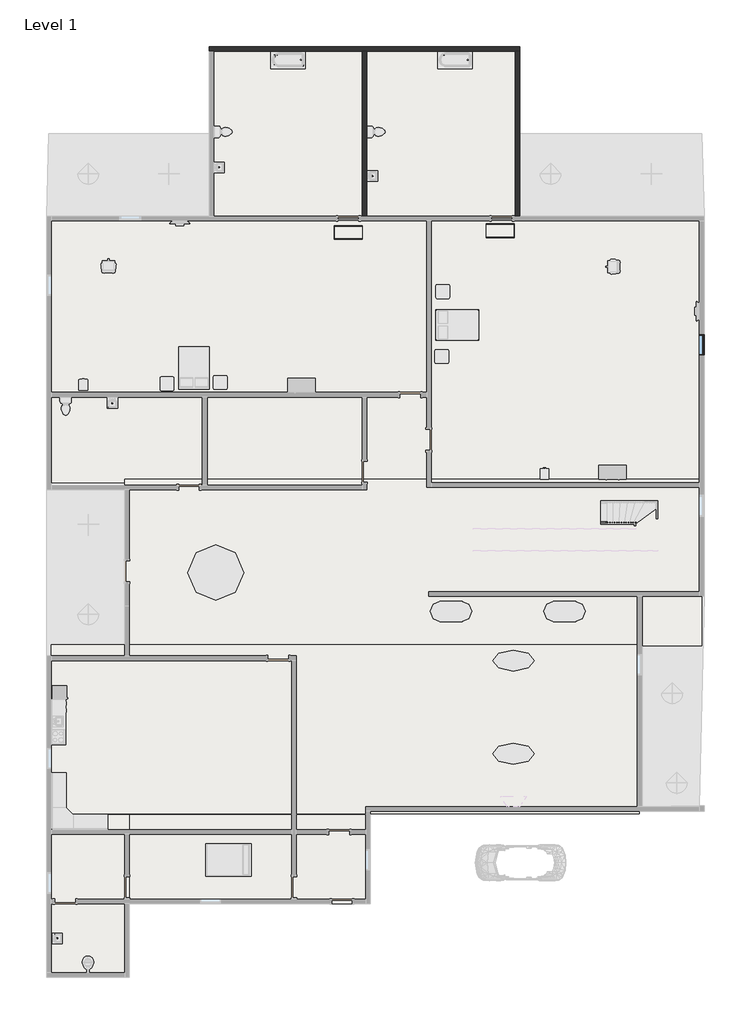
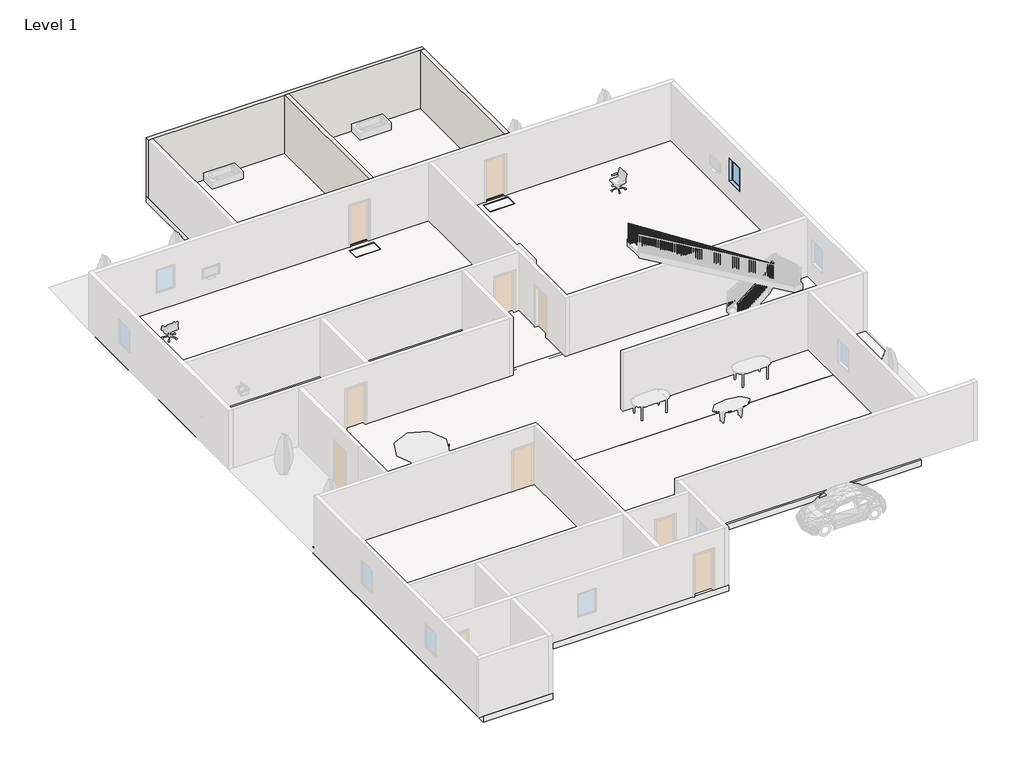
# One storey, part 2 of 4: 7 slabs, 3 walls, 1 railing, 1 window.
"""IFC4 building model written with IfcOpenShell, lengths in millimetres."""

from ifc_helpers import new_model, si_unit, frame, origin, origin_with_axes, place, context, project, spatial, polyline, outline, extrude, faceted_brep, transform, mapped, element, save
from components import window_e2841890

model = new_model("IFC4")

# Units and contexts
model_context = context("Model", 3, world=origin())
ifc_project = project(units=[si_unit("LENGTHUNIT", "METRE", prefix="MILLI")], contexts=[model_context])

# Site, building, storey
site = spatial("IfcSite", under=ifc_project)
building = spatial("IfcBuilding", under=site)
storey = spatial("IfcBuildingStorey", under=building, Name="Level 1", Elevation=0.0)

# Railing
placement = place(None, origin())
element("IfcRailing", 1, ObjectType="Handrail - Rectangular", at=placement, inside=storey, context=model_context, shape_type="SolidModel", body=[
    faceted_brep([(11576.2992414, 107.8275916, 1025.2529681), (11576.2992414, 107.8275916, 959.7067088), (11576.2992414, 57.0275916, 959.7067088), (11576.2992414, 57.0275916, 1025.2529681), (13027.8309332, 107.8275916, 2208.7848338), (13078.6309332, 107.8275916, 2184.659247), (13078.6309332, 57.0275916, 2184.659247), (13027.8309332, 57.0275916, 2208.7848338), (13027.8309332, 107.8275916, 2414.6281882), (13078.6309332, 107.8275916, 2363.8281882), (13078.6309332, 57.0275916, 2363.8281882), (13027.8309332, 57.0275916, 2414.6281882), (13154.8309332, 107.8275916, 2414.6281882), (13154.8309332, 107.8275916, 2363.8281882), (13104.0309332, 57.0275916, 2363.8281882), (13104.0309332, 57.0275916, 2414.6281882), (13154.8309332, -19.1724084, 2414.6281882), (13154.8309332, -48.2937422, 2363.8281882), (13104.0309332, -48.2937422, 2363.8281882), (13104.0309332, -19.1724084, 2414.6281882), (13154.8309332, -146.1724084, 2631.5051451), (13154.8309332, -196.9724084, 2617.7256424), (13104.0309332, -196.9724084, 2617.7256424), (13104.0309332, -146.1724084, 2631.5051451), (13154.8309332, -146.1724084, 2824.6954835), (13154.8309332, -196.9724084, 2773.8954835), (13104.0309332, -196.9724084, 2773.8954835), (13104.0309332, -146.1724084, 2824.6954835), (13154.8309332, -273.1724084, 2824.6954835), (13154.8309332, -273.1724084, 2773.8954835), (13104.0309332, -222.3724084, 2773.8954835), (13104.0309332, -222.3724084, 2824.6954835), (13027.8309332, -273.1724084, 2824.6954835), (13012.8842088, -273.1724084, 2773.8954835), (13012.8842088, -222.3724084, 2773.8954835), (13027.8309332, -222.3724084, 2824.6954835), (5988.2992414, -273.1724084, 7359.7294681), (5988.2992414, -222.3724084, 7359.7294681), (5988.2992414, -222.3724084, 7299.3004322), (5988.2992414, -273.1724084, 7299.3004322)], [[[0, 1, 2, 3]], [[1, 0, 4, 5]], [[2, 1, 5, 6]], [[3, 2, 6, 7]], [[0, 3, 7, 4]], [[5, 4, 8, 9]], [[6, 5, 9, 10]], [[7, 6, 10, 11]], [[4, 7, 11, 8]], [[9, 8, 12, 13]], [[10, 9, 13, 14]], [[11, 10, 14, 15]], [[8, 11, 15, 12]], [[13, 12, 16, 17]], [[14, 13, 17, 18]], [[15, 14, 18, 19]], [[12, 15, 19, 16]], [[17, 16, 20, 21]], [[18, 17, 21, 22]], [[19, 18, 22, 23]], [[16, 19, 23, 20]], [[21, 20, 24, 25]], [[22, 21, 25, 26]], [[23, 22, 26, 27]], [[20, 23, 27, 24]], [[25, 24, 28, 29]], [[26, 25, 29, 30]], [[27, 26, 30, 31]], [[24, 27, 31, 28]], [[29, 28, 32, 33]], [[30, 29, 33, 34]], [[31, 30, 34, 35]], [[28, 31, 35, 32]], [[36, 37, 38, 39]], [[33, 32, 36, 39]], [[34, 33, 39, 38]], [[35, 34, 38, 37]], [[32, 35, 37, 36]]]),
    extrude(outline(polyline([(7231.8259142, 6093.0369367), (7244.098378, 6073.9869367), (6265.3333333, 6073.9869367), (6265.3333333, 6093.0369367), (7231.8259142, 6093.0369367)])), frame((0.0, -257.2974084, 0.0), z_axis=(0.0, 1.0, 0.0), x_axis=(0.0, 0.0, 1.0)), (0.0, 0.0, 1.0), 19.05),
    extrude(outline(polyline([(7166.3727743, 6194.6369367), (7178.645238, 6175.5869367), (6265.3333333, 6175.5869367), (6265.3333333, 6194.6369367), (7166.3727743, 6194.6369367)])), frame((0.0, -257.2974084, 0.0), z_axis=(0.0, 1.0, 0.0), x_axis=(0.0, 0.0, 1.0)), (0.0, 0.0, 1.0), 19.05),
    extrude(outline(polyline([(7100.9196344, 6296.2369367), (7113.1920981, 6277.1869367), (6096.0, 6277.1869367), (6096.0, 6296.2369367), (7100.9196344, 6296.2369367)])), frame((0.0, -257.2974084, 0.0), z_axis=(0.0, 1.0, 0.0), x_axis=(0.0, 0.0, 1.0)), (0.0, 0.0, 1.0), 19.05),
    extrude(outline(polyline([(7035.4664945, 6397.8369367), (7047.7389582, 6378.7869367), (6096.0, 6378.7869367), (6096.0, 6397.8369367), (7035.4664945, 6397.8369367)])), frame((0.0, -257.2974084, 0.0), z_axis=(0.0, 1.0, 0.0), x_axis=(0.0, 0.0, 1.0)), (0.0, 0.0, 1.0), 19.05),
    extrude(outline(polyline([(6970.0133545, 6499.4369367), (6982.2858183, 6480.3869367), (6096.0, 6480.3869367), (6096.0, 6499.4369367), (6970.0133545, 6499.4369367)])), frame((0.0, -257.2974084, 0.0), z_axis=(0.0, 1.0, 0.0), x_axis=(0.0, 0.0, 1.0)), (0.0, 0.0, 1.0), 19.05),
    extrude(outline(polyline([(6904.5602146, 6601.0369367), (6916.8326783, 6581.9869367), (5926.6666667, 6581.9869367), (5926.6666667, 6601.0369367), (6904.5602146, 6601.0369367)])), frame((0.0, -257.2974084, 0.0), z_axis=(0.0, 1.0, 0.0), x_axis=(0.0, 0.0, 1.0)), (0.0, 0.0, 1.0), 19.05),
    extrude(outline(polyline([(6839.1070747, 6702.6369367), (6851.3795384, 6683.5869367), (5926.6666667, 6683.5869367), (5926.6666667, 6702.6369367), (6839.1070747, 6702.6369367)])), frame((0.0, -257.2974084, 0.0), z_axis=(0.0, 1.0, 0.0), x_axis=(0.0, 0.0, 1.0)), (0.0, 0.0, 1.0), 19.05),
    extrude(outline(polyline([(6773.6539348, 6804.2369367), (6785.9263985, 6785.1869367), (5926.6666667, 6785.1869367), (5926.6666667, 6804.2369367), (6773.6539348, 6804.2369367)])), frame((0.0, -257.2974084, 0.0), z_axis=(0.0, 1.0, 0.0), x_axis=(0.0, 0.0, 1.0)), (0.0, 0.0, 1.0), 19.05),
    extrude(outline(polyline([(6708.2007948, 6905.8369367), (6720.4732586, 6886.7869367), (5757.3333333, 6886.7869367), (5757.3333333, 6905.8369367), (6708.2007948, 6905.8369367)])), frame((0.0, -257.2974084, 0.0), z_axis=(0.0, 1.0, 0.0), x_axis=(0.0, 0.0, 1.0)), (0.0, 0.0, 1.0), 19.05),
    extrude(outline(polyline([(6642.7476549, 7007.4369367), (6655.0201186, 6988.3869367), (5757.3333333, 6988.3869367), (5757.3333333, 7007.4369367), (6642.7476549, 7007.4369367)])), frame((0.0, -257.2974084, 0.0), z_axis=(0.0, 1.0, 0.0), x_axis=(0.0, 0.0, 1.0)), (0.0, 0.0, 1.0), 19.05),
    extrude(outline(polyline([(6577.294515, 7109.0369367), (6589.5669787, 7089.9869367), (5757.3333333, 7089.9869367), (5757.3333333, 7109.0369367), (6577.294515, 7109.0369367)])), frame((0.0, -257.2974084, 0.0), z_axis=(0.0, 1.0, 0.0), x_axis=(0.0, 0.0, 1.0)), (0.0, 0.0, 1.0), 19.05),
    extrude(outline(polyline([(6511.8413751, 7210.6369367), (6524.1138388, 7191.5869367), (5588.0, 7191.5869367), (5588.0, 7210.6369367), (6511.8413751, 7210.6369367)])), frame((0.0, -257.2974084, 0.0), z_axis=(0.0, 1.0, 0.0), x_axis=(0.0, 0.0, 1.0)), (0.0, 0.0, 1.0), 19.05),
    extrude(outline(polyline([(6446.3882351, 7312.2369367), (6458.6606989, 7293.1869367), (5588.0, 7293.1869367), (5588.0, 7312.2369367), (6446.3882351, 7312.2369367)])), frame((0.0, -257.2974084, 0.0), z_axis=(0.0, 1.0, 0.0), x_axis=(0.0, 0.0, 1.0)), (0.0, 0.0, 1.0), 19.05),
    extrude(outline(polyline([(6380.9350952, 7413.8369367), (6393.2075589, 7394.7869367), (5418.6666667, 7394.7869367), (5418.6666667, 7413.8369367), (6380.9350952, 7413.8369367)])), frame((0.0, -257.2974084, 0.0), z_axis=(0.0, 1.0, 0.0), x_axis=(0.0, 0.0, 1.0)), (0.0, 0.0, 1.0), 19.05),
    extrude(outline(polyline([(6315.4819553, 7515.4369367), (6327.754419, 7496.3869367), (5418.6666667, 7496.3869367), (5418.6666667, 7515.4369367), (6315.4819553, 7515.4369367)])), frame((0.0, -257.2974084, 0.0), z_axis=(0.0, 1.0, 0.0), x_axis=(0.0, 0.0, 1.0)), (0.0, 0.0, 1.0), 19.05),
    extrude(outline(polyline([(6250.0288153, 7617.0369367), (6262.3012791, 7597.9869367), (5418.6666667, 7597.9869367), (5418.6666667, 7617.0369367), (6250.0288153, 7617.0369367)])), frame((0.0, -257.2974084, 0.0), z_axis=(0.0, 1.0, 0.0), x_axis=(0.0, 0.0, 1.0)), (0.0, 0.0, 1.0), 19.05),
    extrude(outline(polyline([(6184.5756754, 7718.6369367), (6196.8481392, 7699.5869367), (5249.3333333, 7699.5869367), (5249.3333333, 7718.6369367), (6184.5756754, 7718.6369367)])), frame((0.0, -257.2974084, 0.0), z_axis=(0.0, 1.0, 0.0), x_axis=(0.0, 0.0, 1.0)), (0.0, 0.0, 1.0), 19.05),
    extrude(outline(polyline([(6119.1225355, 7820.2369367), (6131.3949992, 7801.1869367), (5249.3333333, 7801.1869367), (5249.3333333, 7820.2369367), (6119.1225355, 7820.2369367)])), frame((0.0, -257.2974084, 0.0), z_axis=(0.0, 1.0, 0.0), x_axis=(0.0, 0.0, 1.0)), (0.0, 0.0, 1.0), 19.05),
    extrude(outline(polyline([(6053.6693956, 7921.8369367), (6065.9418593, 7902.7869367), (5249.3333333, 7902.7869367), (5249.3333333, 7921.8369367), (6053.6693956, 7921.8369367)])), frame((0.0, -257.2974084, 0.0), z_axis=(0.0, 1.0, 0.0), x_axis=(0.0, 0.0, 1.0)), (0.0, 0.0, 1.0), 19.05),
    extrude(outline(polyline([(5988.2162556, 8023.4369367), (6000.4887194, 8004.3869367), (5080.0, 8004.3869367), (5080.0, 8023.4369367), (5988.2162556, 8023.4369367)])), frame((0.0, -257.2974084, 0.0), z_axis=(0.0, 1.0, 0.0), x_axis=(0.0, 0.0, 1.0)), (0.0, 0.0, 1.0), 19.05),
    extrude(outline(polyline([(5922.7631157, 8125.0369367), (5935.0355795, 8105.9869367), (5080.0, 8105.9869367), (5080.0, 8125.0369367), (5922.7631157, 8125.0369367)])), frame((0.0, -257.2974084, 0.0), z_axis=(0.0, 1.0, 0.0), x_axis=(0.0, 0.0, 1.0)), (0.0, 0.0, 1.0), 19.05),
    extrude(outline(polyline([(5857.3099758, 8226.6369367), (5869.5824395, 8207.5869367), (5080.0, 8207.5869367), (5080.0, 8226.6369367), (5857.3099758, 8226.6369367)])), frame((0.0, -257.2974084, 0.0), z_axis=(0.0, 1.0, 0.0), x_axis=(0.0, 0.0, 1.0)), (0.0, 0.0, 1.0), 19.05),
    extrude(outline(polyline([(5791.8568359, 8328.2369367), (5804.1292996, 8309.1869367), (4910.6666667, 8309.1869367), (4910.6666667, 8328.2369367), (5791.8568359, 8328.2369367)])), frame((0.0, -257.2974084, 0.0), z_axis=(0.0, 1.0, 0.0), x_axis=(0.0, 0.0, 1.0)), (0.0, 0.0, 1.0), 19.05),
    extrude(outline(polyline([(5726.4036959, 8429.8369367), (5738.6761597, 8410.7869367), (4910.6666667, 8410.7869367), (4910.6666667, 8429.8369367), (5726.4036959, 8429.8369367)])), frame((0.0, -257.2974084, 0.0), z_axis=(0.0, 1.0, 0.0), x_axis=(0.0, 0.0, 1.0)), (0.0, 0.0, 1.0), 19.05),
    extrude(outline(polyline([(5660.950556, 8531.4369367), (5673.2230198, 8512.3869367), (4741.3333333, 8512.3869367), (4741.3333333, 8531.4369367), (5660.950556, 8531.4369367)])), frame((0.0, -257.2974084, 0.0), z_axis=(0.0, 1.0, 0.0), x_axis=(0.0, 0.0, 1.0)), (0.0, 0.0, 1.0), 19.05),
    extrude(outline(polyline([(5595.4974161, 8633.0369367), (5607.7698798, 8613.9869367), (4741.3333333, 8613.9869367), (4741.3333333, 8633.0369367), (5595.4974161, 8633.0369367)])), frame((0.0, -257.2974084, 0.0), z_axis=(0.0, 1.0, 0.0), x_axis=(0.0, 0.0, 1.0)), (0.0, 0.0, 1.0), 19.05),
    extrude(outline(polyline([(5530.0442762, 8734.6369367), (5542.3167399, 8715.5869367), (4741.3333333, 8715.5869367), (4741.3333333, 8734.6369367), (5530.0442762, 8734.6369367)])), frame((0.0, -257.2974084, 0.0), z_axis=(0.0, 1.0, 0.0), x_axis=(0.0, 0.0, 1.0)), (0.0, 0.0, 1.0), 19.05),
    extrude(outline(polyline([(5464.5911362, 8836.2369367), (5476.8636, 8817.1869367), (4572.0, 8817.1869367), (4572.0, 8836.2369367), (5464.5911362, 8836.2369367)])), frame((0.0, -257.2974084, 0.0), z_axis=(0.0, 1.0, 0.0), x_axis=(0.0, 0.0, 1.0)), (0.0, 0.0, 1.0), 19.05),
    extrude(outline(polyline([(5399.1379963, 8937.8369367), (5411.41046, 8918.7869367), (4572.0, 8918.7869367), (4572.0, 8937.8369367), (5399.1379963, 8937.8369367)])), frame((0.0, -257.2974084, 0.0), z_axis=(0.0, 1.0, 0.0), x_axis=(0.0, 0.0, 1.0)), (0.0, 0.0, 1.0), 19.05),
    extrude(outline(polyline([(5333.6848564, 9039.4369367), (5345.9573201, 9020.3869367), (4572.0, 9020.3869367), (4572.0, 9039.4369367), (5333.6848564, 9039.4369367)])), frame((0.0, -257.2974084, 0.0), z_axis=(0.0, 1.0, 0.0), x_axis=(0.0, 0.0, 1.0)), (0.0, 0.0, 1.0), 19.05),
    extrude(outline(polyline([(5268.2317165, 9141.0369367), (5280.5041802, 9121.9869367), (4402.6666667, 9121.9869367), (4402.6666667, 9141.0369367), (5268.2317165, 9141.0369367)])), frame((0.0, -257.2974084, 0.0), z_axis=(0.0, 1.0, 0.0), x_axis=(0.0, 0.0, 1.0)), (0.0, 0.0, 1.0), 19.05),
    extrude(outline(polyline([(5202.7785765, 9242.6369367), (5215.0510403, 9223.5869367), (4402.6666667, 9223.5869367), (4402.6666667, 9242.6369367), (5202.7785765, 9242.6369367)])), frame((0.0, -257.2974084, 0.0), z_axis=(0.0, 1.0, 0.0), x_axis=(0.0, 0.0, 1.0)), (0.0, 0.0, 1.0), 19.05),
    extrude(outline(polyline([(5137.3254366, 9344.2369367), (5149.5979003, 9325.1869367), (4233.3333333, 9325.1869367), (4233.3333333, 9344.2369367), (5137.3254366, 9344.2369367)])), frame((0.0, -257.2974084, 0.0), z_axis=(0.0, 1.0, 0.0), x_axis=(0.0, 0.0, 1.0)), (0.0, 0.0, 1.0), 19.05),
    extrude(outline(polyline([(5071.8722967, 9445.8369367), (5084.1447604, 9426.7869367), (4233.3333333, 9426.7869367), (4233.3333333, 9445.8369367), (5071.8722967, 9445.8369367)])), frame((0.0, -257.2974084, 0.0), z_axis=(0.0, 1.0, 0.0), x_axis=(0.0, 0.0, 1.0)), (0.0, 0.0, 1.0), 19.05),
    extrude(outline(polyline([(5006.4191568, 9547.4369367), (5018.6916205, 9528.3869367), (4233.3333333, 9528.3869367), (4233.3333333, 9547.4369367), (5006.4191568, 9547.4369367)])), frame((0.0, -257.2974084, 0.0), z_axis=(0.0, 1.0, 0.0), x_axis=(0.0, 0.0, 1.0)), (0.0, 0.0, 1.0), 19.05),
    extrude(outline(polyline([(4940.9660168, 9649.0369367), (4953.2384806, 9629.9869367), (4064.0, 9629.9869367), (4064.0, 9649.0369367), (4940.9660168, 9649.0369367)])), frame((0.0, -257.2974084, 0.0), z_axis=(0.0, 1.0, 0.0), x_axis=(0.0, 0.0, 1.0)), (0.0, 0.0, 1.0), 19.05),
    extrude(outline(polyline([(4875.5128769, 9750.6369367), (4887.7853406, 9731.5869367), (4064.0, 9731.5869367), (4064.0, 9750.6369367), (4875.5128769, 9750.6369367)])), frame((0.0, -257.2974084, 0.0), z_axis=(0.0, 1.0, 0.0), x_axis=(0.0, 0.0, 1.0)), (0.0, 0.0, 1.0), 19.05),
    extrude(outline(polyline([(4810.059737, 9852.2369367), (4822.3322007, 9833.1869367), (4064.0, 9833.1869367), (4064.0, 9852.2369367), (4810.059737, 9852.2369367)])), frame((0.0, -257.2974084, 0.0), z_axis=(0.0, 1.0, 0.0), x_axis=(0.0, 0.0, 1.0)), (0.0, 0.0, 1.0), 19.05),
    extrude(outline(polyline([(4744.6065971, 9953.8369367), (4756.8790608, 9934.7869367), (3894.6666667, 9934.7869367), (3894.6666667, 9953.8369367), (4744.6065971, 9953.8369367)])), frame((0.0, -257.2974084, 0.0), z_axis=(0.0, 1.0, 0.0), x_axis=(0.0, 0.0, 1.0)), (0.0, 0.0, 1.0), 19.05),
    extrude(outline(polyline([(4679.1534571, 10055.4369367), (4691.4259209, 10036.3869367), (3894.6666667, 10036.3869367), (3894.6666667, 10055.4369367), (4679.1534571, 10055.4369367)])), frame((0.0, -257.2974084, 0.0), z_axis=(0.0, 1.0, 0.0), x_axis=(0.0, 0.0, 1.0)), (0.0, 0.0, 1.0), 19.05),
    extrude(outline(polyline([(4613.7003172, 10157.0369367), (4625.9727809, 10137.9869367), (3894.6666667, 10137.9869367), (3894.6666667, 10157.0369367), (4613.7003172, 10157.0369367)])), frame((0.0, -257.2974084, 0.0), z_axis=(0.0, 1.0, 0.0), x_axis=(0.0, 0.0, 1.0)), (0.0, 0.0, 1.0), 19.05),
    extrude(outline(polyline([(4548.2471773, 10258.6369367), (4560.519641, 10239.5869367), (3725.3333333, 10239.5869367), (3725.3333333, 10258.6369367), (4548.2471773, 10258.6369367)])), frame((0.0, -257.2974084, 0.0), z_axis=(0.0, 1.0, 0.0), x_axis=(0.0, 0.0, 1.0)), (0.0, 0.0, 1.0), 19.05),
    extrude(outline(polyline([(4482.7940373, 10360.2369367), (4495.0665011, 10341.1869367), (3725.3333333, 10341.1869367), (3725.3333333, 10360.2369367), (4482.7940373, 10360.2369367)])), frame((0.0, -257.2974084, 0.0), z_axis=(0.0, 1.0, 0.0), x_axis=(0.0, 0.0, 1.0)), (0.0, 0.0, 1.0), 19.05),
    extrude(outline(polyline([(4417.3408974, 10461.8369367), (4429.6133612, 10442.7869367), (3556.0, 10442.7869367), (3556.0, 10461.8369367), (4417.3408974, 10461.8369367)])), frame((0.0, -257.2974084, 0.0), z_axis=(0.0, 1.0, 0.0), x_axis=(0.0, 0.0, 1.0)), (0.0, 0.0, 1.0), 19.05),
    extrude(outline(polyline([(4351.8877575, 10563.4369367), (4364.1602212, 10544.3869367), (3556.0, 10544.3869367), (3556.0, 10563.4369367), (4351.8877575, 10563.4369367)])), frame((0.0, -257.2974084, 0.0), z_axis=(0.0, 1.0, 0.0), x_axis=(0.0, 0.0, 1.0)), (0.0, 0.0, 1.0), 19.05),
    extrude(outline(polyline([(4286.4346176, 10665.0369367), (4298.7070813, 10645.9869367), (3556.0, 10645.9869367), (3556.0, 10665.0369367), (4286.4346176, 10665.0369367)])), frame((0.0, -257.2974084, 0.0), z_axis=(0.0, 1.0, 0.0), x_axis=(0.0, 0.0, 1.0)), (0.0, 0.0, 1.0), 19.05),
    extrude(outline(polyline([(4220.9814776, 10766.6369367), (4233.2539414, 10747.5869367), (3386.6666667, 10747.5869367), (3386.6666667, 10766.6369367), (4220.9814776, 10766.6369367)])), frame((0.0, -257.2974084, 0.0), z_axis=(0.0, 1.0, 0.0), x_axis=(0.0, 0.0, 1.0)), (0.0, 0.0, 1.0), 19.05),
    extrude(outline(polyline([(4155.5283377, 10868.2369367), (4167.8008015, 10849.1869367), (3386.6666667, 10849.1869367), (3386.6666667, 10868.2369367), (4155.5283377, 10868.2369367)])), frame((0.0, -257.2974084, 0.0), z_axis=(0.0, 1.0, 0.0), x_axis=(0.0, 0.0, 1.0)), (0.0, 0.0, 1.0), 19.05),
    extrude(outline(polyline([(4090.0751978, 10969.8369367), (4102.3476615, 10950.7869367), (3386.6666667, 10950.7869367), (3386.6666667, 10969.8369367), (4090.0751978, 10969.8369367)])), frame((0.0, -257.2974084, 0.0), z_axis=(0.0, 1.0, 0.0), x_axis=(0.0, 0.0, 1.0)), (0.0, 0.0, 1.0), 19.05),
    extrude(outline(polyline([(4024.6220579, 11071.4369367), (4036.8945216, 11052.3869367), (3217.3333333, 11052.3869367), (3217.3333333, 11071.4369367), (4024.6220579, 11071.4369367)])), frame((0.0, -257.2974084, 0.0), z_axis=(0.0, 1.0, 0.0), x_axis=(0.0, 0.0, 1.0)), (0.0, 0.0, 1.0), 19.05),
    extrude(outline(polyline([(3959.1689179, 11173.0369367), (3971.4413817, 11153.9869367), (3217.3333333, 11153.9869367), (3217.3333333, 11173.0369367), (3959.1689179, 11173.0369367)])), frame((0.0, -257.2974084, 0.0), z_axis=(0.0, 1.0, 0.0), x_axis=(0.0, 0.0, 1.0)), (0.0, 0.0, 1.0), 19.05),
    extrude(outline(polyline([(3893.715778, 11274.6369367), (3905.9882418, 11255.5869367), (3217.3333333, 11255.5869367), (3217.3333333, 11274.6369367), (3893.715778, 11274.6369367)])), frame((0.0, -257.2974084, 0.0), z_axis=(0.0, 1.0, 0.0), x_axis=(0.0, 0.0, 1.0)), (0.0, 0.0, 1.0), 19.05),
    extrude(outline(polyline([(3828.2626381, 11376.2369367), (3840.5351018, 11357.1869367), (3048.0, 11357.1869367), (3048.0, 11376.2369367), (3828.2626381, 11376.2369367)])), frame((0.0, -257.2974084, 0.0), z_axis=(0.0, 1.0, 0.0), x_axis=(0.0, 0.0, 1.0)), (0.0, 0.0, 1.0), 19.05),
    extrude(outline(polyline([(3762.8094982, 11477.8369367), (3775.0819619, 11458.7869367), (3048.0, 11458.7869367), (3048.0, 11477.8369367), (3762.8094982, 11477.8369367)])), frame((0.0, -257.2974084, 0.0), z_axis=(0.0, 1.0, 0.0), x_axis=(0.0, 0.0, 1.0)), (0.0, 0.0, 1.0), 19.05),
    extrude(outline(polyline([(3697.3563582, 11579.4369367), (3709.628822, 11560.3869367), (2878.6666667, 11560.3869367), (2878.6666667, 11579.4369367), (3697.3563582, 11579.4369367)])), frame((0.0, -257.2974084, 0.0), z_axis=(0.0, 1.0, 0.0), x_axis=(0.0, 0.0, 1.0)), (0.0, 0.0, 1.0), 19.05),
    extrude(outline(polyline([(3631.9032183, 11681.0369367), (3644.175682, 11661.9869367), (2878.6666667, 11661.9869367), (2878.6666667, 11681.0369367), (3631.9032183, 11681.0369367)])), frame((0.0, -257.2974084, 0.0), z_axis=(0.0, 1.0, 0.0), x_axis=(0.0, 0.0, 1.0)), (0.0, 0.0, 1.0), 19.05),
    extrude(outline(polyline([(3566.4500784, 11782.6369367), (3578.7225421, 11763.5869367), (2878.6666667, 11763.5869367), (2878.6666667, 11782.6369367), (3566.4500784, 11782.6369367)])), frame((0.0, -257.2974084, 0.0), z_axis=(0.0, 1.0, 0.0), x_axis=(0.0, 0.0, 1.0)), (0.0, 0.0, 1.0), 19.05),
    extrude(outline(polyline([(3500.9969385, 11884.2369367), (3513.2694022, 11865.1869367), (2709.3333333, 11865.1869367), (2709.3333333, 11884.2369367), (3500.9969385, 11884.2369367)])), frame((0.0, -257.2974084, 0.0), z_axis=(0.0, 1.0, 0.0), x_axis=(0.0, 0.0, 1.0)), (0.0, 0.0, 1.0), 19.05),
    extrude(outline(polyline([(3435.5437985, 11985.8369367), (3447.8162623, 11966.7869367), (2709.3333333, 11966.7869367), (2709.3333333, 11985.8369367), (3435.5437985, 11985.8369367)])), frame((0.0, -257.2974084, 0.0), z_axis=(0.0, 1.0, 0.0), x_axis=(0.0, 0.0, 1.0)), (0.0, 0.0, 1.0), 19.05),
    extrude(outline(polyline([(3370.0906586, 12087.4369367), (3382.3631223, 12068.3869367), (2709.3333333, 12068.3869367), (2709.3333333, 12087.4369367), (3370.0906586, 12087.4369367)])), frame((0.0, -257.2974084, 0.0), z_axis=(0.0, 1.0, 0.0), x_axis=(0.0, 0.0, 1.0)), (0.0, 0.0, 1.0), 19.05),
    extrude(outline(polyline([(3304.6375187, 12189.0369367), (3316.9099824, 12169.9869367), (2540.0, 12169.9869367), (2540.0, 12189.0369367), (3304.6375187, 12189.0369367)])), frame((0.0, -257.2974084, 0.0), z_axis=(0.0, 1.0, 0.0), x_axis=(0.0, 0.0, 1.0)), (0.0, 0.0, 1.0), 19.05),
    extrude(outline(polyline([(3239.1843788, 12290.6369367), (3251.4568425, 12271.5869367), (2540.0, 12271.5869367), (2540.0, 12290.6369367), (3239.1843788, 12290.6369367)])), frame((0.0, -257.2974084, 0.0), z_axis=(0.0, 1.0, 0.0), x_axis=(0.0, 0.0, 1.0)), (0.0, 0.0, 1.0), 19.05),
    extrude(outline(polyline([(3173.7312388, 12392.2369367), (3186.0037026, 12373.1869367), (2370.6666667, 12373.1869367), (2370.6666667, 12392.2369367), (3173.7312388, 12392.2369367)])), frame((0.0, -257.2974084, 0.0), z_axis=(0.0, 1.0, 0.0), x_axis=(0.0, 0.0, 1.0)), (0.0, 0.0, 1.0), 19.05),
    extrude(outline(polyline([(3108.2780989, 12493.8369367), (3120.5505626, 12474.7869367), (2370.6666667, 12474.7869367), (2370.6666667, 12493.8369367), (3108.2780989, 12493.8369367)])), frame((0.0, -257.2974084, 0.0), z_axis=(0.0, 1.0, 0.0), x_axis=(0.0, 0.0, 1.0)), (0.0, 0.0, 1.0), 19.05),
    extrude(outline(polyline([(3042.824959, 12595.4369367), (3055.0974227, 12576.3869367), (2370.6666667, 12576.3869367), (2370.6666667, 12595.4369367), (3042.824959, 12595.4369367)])), frame((0.0, -257.2974084, 0.0), z_axis=(0.0, 1.0, 0.0), x_axis=(0.0, 0.0, 1.0)), (0.0, 0.0, 1.0), 19.05),
    extrude(outline(polyline([(2977.3718191, 12697.0369367), (2989.6442828, 12677.9869367), (2201.3333333, 12677.9869367), (2201.3333333, 12697.0369367), (2977.3718191, 12697.0369367)])), frame((0.0, -257.2974084, 0.0), z_axis=(0.0, 1.0, 0.0), x_axis=(0.0, 0.0, 1.0)), (0.0, 0.0, 1.0), 19.05),
    extrude(outline(polyline([(2911.9186791, 12798.6369367), (2924.1911429, 12779.5869367), (2201.3333333, 12779.5869367), (2201.3333333, 12798.6369367), (2911.9186791, 12798.6369367)])), frame((0.0, -257.2974084, 0.0), z_axis=(0.0, 1.0, 0.0), x_axis=(0.0, 0.0, 1.0)), (0.0, 0.0, 1.0), 19.05),
    extrude(outline(polyline([(2846.4655392, 12900.2369367), (2858.7380029, 12881.1869367), (2032.0, 12881.1869367), (2032.0, 12900.2369367), (2846.4655392, 12900.2369367)])), frame((0.0, -257.2974084, 0.0), z_axis=(0.0, 1.0, 0.0), x_axis=(0.0, 0.0, 1.0)), (0.0, 0.0, 1.0), 19.05),
    extrude(outline(polyline([(2781.0123993, 13001.8369367), (2793.284863, 12982.7869367), (2032.0, 12982.7869367), (2032.0, 13001.8369367), (2781.0123993, 13001.8369367)])), frame((0.0, -257.2974084, 0.0), z_axis=(0.0, 1.0, 0.0), x_axis=(0.0, 0.0, 1.0)), (0.0, 0.0, 1.0), 19.05),
    extrude(outline(polyline([(-145.0833121, 2529.115018), (-126.0333121, 2496.5834745), (-126.0333121, 1524.0), (-145.0833121, 1524.0), (-145.0833121, 2529.115018)])), frame((13119.9059332, 0.0, 0.0), z_axis=(1.0, 0.0, 0.0), x_axis=(0.0, 1.0, 0.0)), (0.0, 0.0, 1.0), 19.05),
    extrude(outline(polyline([(-43.4833121, 2355.6134525), (-24.4333121, 2323.0819089), (-24.4333121, 1524.0), (-43.4833121, 1524.0), (-43.4833121, 2355.6134525)])), frame((13119.9059332, 0.0, 0.0), z_axis=(1.0, 0.0, 0.0), x_axis=(0.0, 1.0, 0.0)), (0.0, 0.0, 1.0), 19.05),
    extrude(outline(polyline([(2127.2519138, 13008.2242414), (2111.7191617, 12989.1742414), (1016.0, 12989.1742414), (1016.0, 13008.2242414), (2127.2519138, 13008.2242414)])), frame((0.0, 72.9025916, 0.0), z_axis=(0.0, 1.0, 0.0), x_axis=(0.0, 0.0, 1.0)), (0.0, 0.0, 1.0), 19.05),
    extrude(outline(polyline([(2044.4105689, 12906.6242414), (2028.8778167, 12887.5742414), (1016.0, 12887.5742414), (1016.0, 12906.6242414), (2044.4105689, 12906.6242414)])), frame((0.0, 72.9025916, 0.0), z_axis=(0.0, 1.0, 0.0), x_axis=(0.0, 0.0, 1.0)), (0.0, 0.0, 1.0), 19.05),
    extrude(outline(polyline([(1961.569224, 12805.0242414), (1946.0364718, 12785.9742414), (846.6666667, 12785.9742414), (846.6666667, 12805.0242414), (1961.569224, 12805.0242414)])), frame((0.0, 72.9025916, 0.0), z_axis=(0.0, 1.0, 0.0), x_axis=(0.0, 0.0, 1.0)), (0.0, 0.0, 1.0), 19.05),
    extrude(outline(polyline([(1878.7278791, 12703.4242414), (1863.1951269, 12684.3742414), (846.6666667, 12684.3742414), (846.6666667, 12703.4242414), (1878.7278791, 12703.4242414)])), frame((0.0, 72.9025916, 0.0), z_axis=(0.0, 1.0, 0.0), x_axis=(0.0, 0.0, 1.0)), (0.0, 0.0, 1.0), 19.05),
    extrude(outline(polyline([(1795.8865341, 12601.8242414), (1780.353782, 12582.7742414), (677.3333333, 12582.7742414), (677.3333333, 12601.8242414), (1795.8865341, 12601.8242414)])), frame((0.0, 72.9025916, 0.0), z_axis=(0.0, 1.0, 0.0), x_axis=(0.0, 0.0, 1.0)), (0.0, 0.0, 1.0), 19.05),
    extrude(outline(polyline([(1713.0451892, 12500.2242414), (1697.5124371, 12481.1742414), (677.3333333, 12481.1742414), (677.3333333, 12500.2242414), (1713.0451892, 12500.2242414)])), frame((0.0, 72.9025916, 0.0), z_axis=(0.0, 1.0, 0.0), x_axis=(0.0, 0.0, 1.0)), (0.0, 0.0, 1.0), 19.05),
    extrude(outline(polyline([(1630.2038443, 12398.6242414), (1614.6710921, 12379.5742414), (508.0, 12379.5742414), (508.0, 12398.6242414), (1630.2038443, 12398.6242414)])), frame((0.0, 72.9025916, 0.0), z_axis=(0.0, 1.0, 0.0), x_axis=(0.0, 0.0, 1.0)), (0.0, 0.0, 1.0), 19.05),
    extrude(outline(polyline([(1547.3624994, 12297.0242414), (1531.8297472, 12277.9742414), (508.0, 12277.9742414), (508.0, 12297.0242414), (1547.3624994, 12297.0242414)])), frame((0.0, 72.9025916, 0.0), z_axis=(0.0, 1.0, 0.0), x_axis=(0.0, 0.0, 1.0)), (0.0, 0.0, 1.0), 19.05),
    extrude(outline(polyline([(1464.5211545, 12195.4242414), (1448.9884023, 12176.3742414), (508.0, 12176.3742414), (508.0, 12195.4242414), (1464.5211545, 12195.4242414)])), frame((0.0, 72.9025916, 0.0), z_axis=(0.0, 1.0, 0.0), x_axis=(0.0, 0.0, 1.0)), (0.0, 0.0, 1.0), 19.05),
    extrude(outline(polyline([(1381.6798095, 12093.8242414), (1366.1470574, 12074.7742414), (338.6666667, 12074.7742414), (338.6666667, 12093.8242414), (1381.6798095, 12093.8242414)])), frame((0.0, 72.9025916, 0.0), z_axis=(0.0, 1.0, 0.0), x_axis=(0.0, 0.0, 1.0)), (0.0, 0.0, 1.0), 19.05),
    extrude(outline(polyline([(1298.8384646, 11992.2242414), (1283.3057124, 11973.1742414), (338.6666667, 11973.1742414), (338.6666667, 11992.2242414), (1298.8384646, 11992.2242414)])), frame((0.0, 72.9025916, 0.0), z_axis=(0.0, 1.0, 0.0), x_axis=(0.0, 0.0, 1.0)), (0.0, 0.0, 1.0), 19.05),
    extrude(outline(polyline([(1215.9971197, 11890.6242414), (1200.4643675, 11871.5742414), (338.6666667, 11871.5742414), (338.6666667, 11890.6242414), (1215.9971197, 11890.6242414)])), frame((0.0, 72.9025916, 0.0), z_axis=(0.0, 1.0, 0.0), x_axis=(0.0, 0.0, 1.0)), (0.0, 0.0, 1.0), 19.05),
    extrude(outline(polyline([(1133.1557748, 11789.0242414), (1117.6230226, 11769.9742414), (169.3333333, 11769.9742414), (169.3333333, 11789.0242414), (1133.1557748, 11789.0242414)])), frame((0.0, 72.9025916, 0.0), z_axis=(0.0, 1.0, 0.0), x_axis=(0.0, 0.0, 1.0)), (0.0, 0.0, 1.0), 19.05),
    extrude(outline(polyline([(1050.3144298, 11687.4242414), (1034.7816777, 11668.3742414), (169.3333333, 11668.3742414), (169.3333333, 11687.4242414), (1050.3144298, 11687.4242414)])), frame((0.0, 72.9025916, 0.0), z_axis=(0.0, 1.0, 0.0), x_axis=(0.0, 0.0, 1.0)), (0.0, 0.0, 1.0), 19.05),
    extrude(outline(polyline([(13103.4369367, -238.2474084), (13103.4369367, -257.2974084), (13084.3869367, -257.2974084), (13084.3869367, -238.2474084), (13103.4369367, -238.2474084)])), frame((0.0, 0.0, 1862.6666667), z_axis=(0.0, 0.0, 1.0), x_axis=(1.0, 0.0, 0.0)), (0.0, 0.0, 1.0), 911.2288168),
    extrude(outline(polyline([(13119.9059332, -238.2474084), (13138.9559332, -238.2474084), (13138.9559332, -257.2974084), (13119.9059332, -257.2974084), (13119.9059332, -238.2474084)])), frame((0.0, 0.0, 1862.6666667), z_axis=(0.0, 0.0, 1.0), x_axis=(1.0, 0.0, 0.0)), (0.0, 0.0, 1.0), 911.2288168),
    extrude(outline(polyline([(13119.9059332, -224.8479336), (13138.9559332, -224.8479336), (13138.9559332, -243.8979336), (13119.9059332, -243.8979336), (13119.9059332, -224.8479336)])), frame((0.0, 0.0, 1693.3333333), z_axis=(0.0, 0.0, 1.0), x_axis=(1.0, 0.0, 0.0)), (0.0, 0.0, 1.0), 1080.5621501),
    extrude(outline(polyline([(13119.9059332, 77.1666879), (13138.9559332, 77.1666879), (13138.9559332, 58.1166879), (13119.9059332, 58.1166879), (13119.9059332, 77.1666879)])), frame((0.0, 0.0, 1354.6666667), z_axis=(0.0, 0.0, 1.0), x_axis=(1.0, 0.0, 0.0)), (0.0, 0.0, 1.0), 1009.1615215),
    extrude(outline(polyline([(13119.9059332, 72.9025916), (13119.9059332, 91.9525916), (13138.9559332, 91.9525916), (13138.9559332, 72.9025916), (13119.9059332, 72.9025916)])), frame((0.0, 0.0, 1185.3333333), z_axis=(0.0, 0.0, 1.0), x_axis=(1.0, 0.0, 0.0)), (0.0, 0.0, 1.0), 1178.4948549),
    extrude(outline(polyline([(13088.9385769, 72.9025916), (13088.9385769, 91.9525916), (13107.9885769, 91.9525916), (13107.9885769, 72.9025916), (13088.9385769, 72.9025916)])), frame((0.0, 0.0, 1185.3333333), z_axis=(0.0, 0.0, 1.0), x_axis=(1.0, 0.0, 0.0)), (0.0, 0.0, 1.0), 1178.4948549),
    extrude(outline(polyline([(7287.0279685, 6007.3492414), (7299.3004322, 5988.2992414), (6265.3333333, 5988.2992414), (6265.3333333, 6007.3492414), (7287.0279685, 6007.3492414)])), frame((0.0, -257.2974084, 0.0), z_axis=(0.0, 1.0, 0.0), x_axis=(0.0, 0.0, 1.0)), (0.0, 0.0, 1.0), 19.05),
    extrude(outline(polyline([(975.239461, 11595.3492414), (959.7067088, 11576.2992414), (169.3333333, 11576.2992414), (169.3333333, 11595.3492414), (975.239461, 11595.3492414)])), frame((0.0, 72.9025916, 0.0), z_axis=(0.0, 1.0, 0.0), x_axis=(0.0, 0.0, 1.0)), (0.0, 0.0, 1.0), 19.05),
])

# Slabs
element("IfcSlab", 2, ObjectType="Generic - 12\"", at=placement, inside=storey, context=model_context, shape_type="SweptSolid", body=[
    extrude(outline(polyline([(7929.3171827, 20942.9665396), (7929.3171827, 13399.1665396), (-5583.4828173, 13399.1665396), (-5583.4828173, 20942.9665396), (7929.3171827, 20942.9665396)])), frame((0.0, 0.0, -304.8), z_axis=(0.0, 0.0, 1.0), x_axis=(1.0, 0.0, 0.0)), (0.0, 0.0, 1.0), 304.8),
])
element("IfcSlab", 3, ObjectType="Generic - 12\"", at=placement, inside=storey, context=model_context, shape_type="Brep", body=[
    faceted_brep([(15904.9171827, 13297.5665396, -304.8), (15904.9171827, 1816.7665396, -304.8), (-12517.6828173, 1816.7665396, -304.8), (-12517.6828173, 13297.5665396, -304.8), (15904.9171827, 13297.5665396, 0.0), (-12517.6828173, 13297.5665396, 0.0), (-12517.6828173, 1816.7665396, 0.0), (15904.9171827, 1816.7665396, 0.0), (-97.0828173, 13094.3665396, 0.0), (1122.1171827, 13094.3665396, 0.0), (1122.1171827, 12484.7665396, 0.0), (-97.0828173, 12484.7665396, 0.0), (6557.7171827, 13170.5665396, 0.0), (7776.9171827, 13170.5665396, 0.0), (7776.9171827, 12560.9665396, 0.0), (6557.7171827, 12560.9665396, 0.0), (1122.1171827, 13094.3665396, -25.4), (-97.0828173, 13094.3665396, -25.4), (-97.0828173, 12484.7665396, -25.4), (1122.1171827, 12484.7665396, -25.4), (7776.9171827, 13170.5665396, -25.4), (6557.7171827, 13170.5665396, -25.4), (6557.7171827, 12560.9665396, -25.4), (7776.9171827, 12560.9665396, -25.4)], [[[0, 1, 2, 3]], [[4, 5, 6, 7], [8, 9, 10, 11], [12, 13, 14, 15]], [[1, 0, 4, 7]], [[2, 1, 7, 6]], [[3, 2, 6, 5]], [[0, 3, 5, 4]], [[16, 17, 18, 19]], [[17, 16, 9, 8]], [[18, 17, 8, 11]], [[19, 18, 11, 10]], [[16, 19, 10, 9]], [[20, 21, 22, 23]], [[21, 20, 13, 12]], [[22, 21, 12, 15]], [[23, 22, 15, 14]], [[20, 23, 14, 13]]]),
])
element("IfcSlab", 4, ObjectType="Generic - 12\"", at=placement, inside=storey, context=model_context, shape_type="SweptSolid", body=[
    extrude(outline(polyline([(16006.5171827, 1969.1665396), (16006.5171827, -5320.6334604), (-9291.8828173, -5320.6334604), (-9291.8828173, 1969.1665396), (16006.5171827, 1969.1665396)])), frame((0.0, 0.0, -304.8), z_axis=(0.0, 0.0, 1.0), x_axis=(1.0, 0.0, 0.0)), (0.0, 0.0, 1.0), 304.8),
])
element("IfcSlab", 5, ObjectType="Generic - 12\"", at=placement, inside=storey, context=model_context, shape_type="SweptSolid", body=[
    extrude(outline(polyline([(13263.3171827, -5295.2334604), (13263.3171827, -12686.6334604), (-12517.6828173, -12686.6334604), (-12517.6828173, -5295.2334604), (13263.3171827, -5295.2334604)])), frame((0.0, 0.0, -304.8), z_axis=(0.0, 0.0, 1.0), x_axis=(1.0, 0.0, 0.0)), (0.0, 0.0, 1.0), 304.8),
])
element("IfcSlab", 6, ObjectType="Generic - 12\"", at=placement, inside=storey, context=model_context, shape_type="SweptSolid", body=[
    extrude(outline(polyline([(-9088.6828173, -12737.4334604), (-9088.6828173, -19874.8334604), (-12517.6828173, -19874.8334604), (-12517.6828173, -12737.4334604), (-9088.6828173, -12737.4334604)])), frame((0.0, 0.0, -304.8), z_axis=(0.0, 0.0, 1.0), x_axis=(1.0, 0.0, 0.0)), (0.0, 0.0, 1.0), 304.8),
])
element("IfcSlab", 7, ObjectType="Generic - 12\"", at=placement, inside=storey, context=model_context, shape_type="SweptSolid", body=[
    extrude(outline(polyline([(1477.7171827, -12737.4334604), (1477.7171827, -16649.0334604), (-9088.6828173, -16649.0334604), (-9088.6828173, -12737.4334604), (1477.7171827, -12737.4334604)])), frame((0.0, 0.0, -304.8), z_axis=(0.0, 0.0, 1.0), x_axis=(1.0, 0.0, 0.0)), (0.0, 0.0, 1.0), 304.8),
])
element("IfcSlab", 8, ObjectType="Generic - 12\"", at=placement, inside=storey, context=model_context, shape_type="SweptSolid", body=[
    extrude(outline(polyline([(-1773.4828173, -12737.4334604), (-1773.4828173, -13601.0334604), (-12517.6828173, -13601.0334604), (-12517.6828173, -12737.4334604), (-1773.4828173, -12737.4334604)])), frame((0.0, 0.0, -304.8), z_axis=(0.0, 0.0, 1.0), x_axis=(1.0, 0.0, 0.0)), (0.0, 0.0, 1.0), 304.8),
])

# Walls
element("IfcWall", 9, ObjectType="Generic - 8\"", at=placement, inside=storey, context=model_context, shape_type="Brep", body=[
    faceted_brep([(-5583.4828173, 20739.7665396, 0.0), (-5380.2828173, 20739.7665396, 0.0), (1122.1171827, 20739.7665396, 0.0), (1325.3171827, 20739.7665396, 0.0), (7827.7171827, 20739.7665396, 0.0), (8030.9171827, 20739.7665396, 0.0), (8030.9171827, 20739.7665396, 3048.0), (7827.7171827, 20739.7665396, 3048.0), (1325.3171827, 20739.7665396, 3048.0), (1122.1171827, 20739.7665396, 3048.0), (-5380.2828173, 20739.7665396, 3048.0), (-5583.4828173, 20739.7665396, 3048.0), (-5583.4828173, 20942.9665396, 0.0), (-5583.4828173, 20942.9665396, 3048.0), (8030.9171827, 20942.9665396, 3048.0), (8030.9171827, 20942.9665396, 0.0)], [[[0, 1, 2, 3, 4, 5, 6, 7, 8, 9, 10, 11]], [[12, 13, 14, 15]], [[5, 4, 3, 2, 1, 0, 12, 15]], [[11, 10, 9, 8, 7, 6, 14, 13]], [[0, 11, 13, 12]], [[6, 5, 15, 14]]]),
])
element("IfcWall", 10, ObjectType="Generic - 8\"", at=placement, inside=storey, context=model_context, shape_type="SweptSolid", body=[
    extrude(outline(polyline([(8030.9171827, 20739.7665396), (8030.9171827, 13500.7665396), (7827.7171827, 13500.7665396), (7827.7171827, 20739.7665396), (8030.9171827, 20739.7665396)])), origin_with_axes(), (0.0, 0.0, 1.0), 3048.0),
])
element("IfcWall", 11, ObjectType="Generic - 8\"", at=placement, inside=storey, context=model_context, shape_type="SweptSolid", body=[
    extrude(outline(polyline([(1122.1171827, 13500.7665396), (1122.1171827, 20739.7665396), (1325.3171827, 20739.7665396), (1325.3171827, 13500.7665396), (1122.1171827, 13500.7665396)])), origin_with_axes(), (0.0, 0.0, 1.0), 3048.0),
])

# Window
window_shape = window_e2841890(model_context)
element("IfcWindow", 12, ObjectType="Fixed : 36\" x 48\"", at=placement, inside=storey, context=model_context, shape_type="MappedRepresentation", body=[
    mapped(window_shape, transform((16006.5171827, 7823.8665396, 0.0), x_axis=(0.0, -1.0, 0.0), y_axis=(1.0, 0.0, 0.0), z_axis=(0.0, 0.0, 1.0))),
])

save(model, "model.ifc")

# Revit data of these elements
# Type "Handrail - Rectangular"
#   Assembly Code = "C2010400"
#   built-in parameter 1008612 = 0.0416667 (stored number, unit not read)
#   built-in parameter 1008611 = 0.0416667 (stored number, unit not read)
#   built-in parameter 1008609 = 0.333333 (stored number, unit not read)
#   built-in parameter 1008604 = 0.166667 (stored number, unit not read)
#   built-in parameter 1008603 = 0.166667 (stored number, unit not read)
#   Railing Height = 3' - 0"
#   built-in parameter 1008630 = 2
#   built-in parameter 1008610 = 2
#   built-in parameter 1008618 = Baluster - Square : 3/4"
# Type "Generic - 12\""
#   Assembly Code = "B1010"
#   Function = 0
#   Layers, outside or top first: 1' - 0" no material (function 1)
# Type "Generic - 8\""
#   Assembly Code = "B2010"
#   Layers, outside or top first: 0' - 8" "Brick, Common" (function 1)
# Type "Fixed : 36\" x 48\""
#   Type Mark = "1"
#   Construction Type Id = "GSP4R"
#   Assembly Code = "B2020100"
#   Analytic Construction = "1/8 in Pilkington single glazing"
#   Visual Light Transmittance = 0.9
#   Solar Heat Gain Coefficient = 0.78
#   Heat Transfer Coefficient (U) = 0.6496 BTU/(h·ft²·°F)
#   Height = 4' - 0"
#   Default Sill Height = 3' - 0"
#   Width = 3' - 0"
#   Window Inset = 0' - 0 3/4"
#   Define Thermal Properties by = 1
#   Glass Pane Material = Glass
#   Sash Material = Sash
#   Wall Closure = (empty or 0)
# Element 1 (IfcRailing, "Handrail - Rectangular")
#   Phase Created = New Construction
# Elements 2, 3, 4, 5, 6, 7, 8 (IfcSlab, "Generic - 12\"")
#   Height Offset From Level = 0' - 0"
#   Phase Created = New Construction
#   Materials on its faces: "Default Floor"
# Elements 9, 10, 11 (IfcWall, "Generic - 8\"")
#   Top Offset = 0' - 0"
#   Base Offset = 0' - 0"
#   Unconnected Height = 10' - 0"
#   wall height = 10' - 0"
#   Phase Created = New Construction
#   Base Constraint = Level 1
#   Materials on its faces: "Brick, Common"
# Element 12 (IfcWindow, "Fixed : 36\" x 48\"")
#   Mark = "12"
#   Phase Created = New Construction
#   Materials on its faces: "Sash", "Glass"
# Materials
#   "Brick, Common": class "Masonry", colour RGB 170 98 104, transparency 0, Description = "Common brick", Cost = 0
#   "Glass": class "Glass", colour RGB 0 128 192, transparency 0.75, Description = "Soda Lime Glass", Cost = 0
#   "Sash": class "Wood", colour RGB 224 178 126, transparency 0
#   "Default Floor": colour RGB 128 128 128, transparency 0
